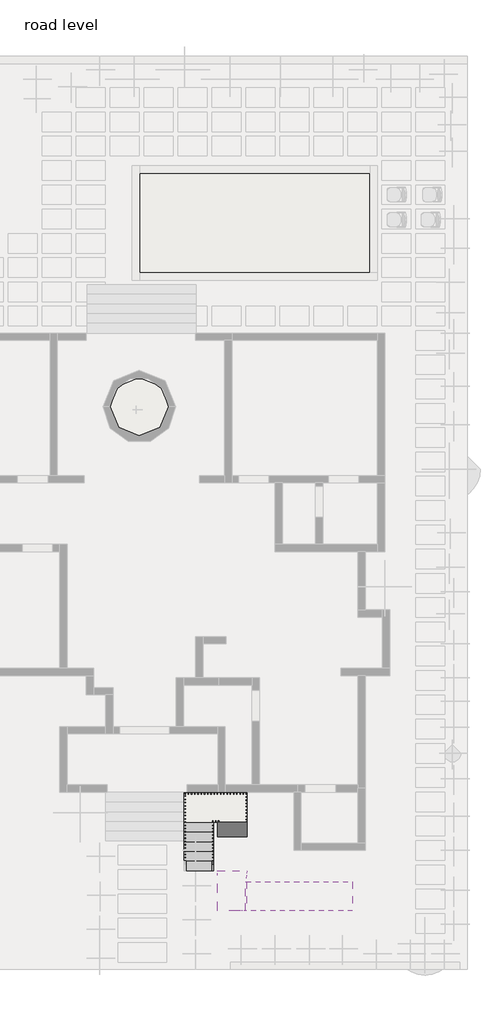
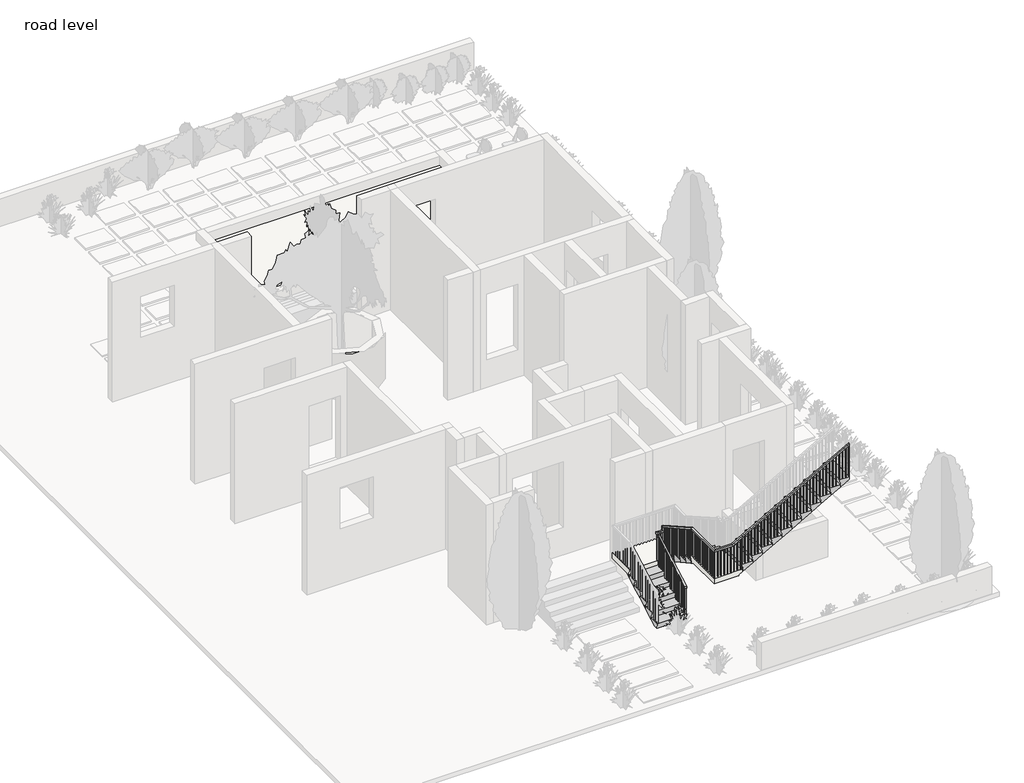
# One storey, part 3 of 5: 7 slabs, 3 stair flights, 1 railing.
"""IFC4 building model written with IfcOpenShell, lengths in millimetres."""

from ifc_helpers import new_model, si_unit, point, frame, frame_2d, origin, origin_with_axes, place, context, project, spatial, polyline, circle_curve, trimmed, segment, composite_curve, outline, extrude, faceted_brep, element, save

model = new_model("IFC4")

# Units and contexts
model_context = context("Model", 3, world=origin())
ifc_project = project(units=[si_unit("LENGTHUNIT", "METRE", prefix="MILLI")], contexts=[model_context])

# Site, building, storey
site = spatial("IfcSite", under=ifc_project)
building = spatial("IfcBuilding", under=site)
storey = spatial("IfcBuildingStorey", under=building, Name="road level", Elevation=0.0)

# Railing
placement = place(None, origin())
element("IfcRailing", 1, ObjectType="Handrail - Rectangular", at=placement, inside=storey, context=model_context, shape_type="SolidModel", body=[
    faceted_brep([(7041.6083823, -2332.334977, 1085.85), (7041.6083823, -2332.334977, 1027.5647478), (7092.4083823, -2332.334977, 1027.5647478), (7092.4083823, -2332.334977, 1085.85), (7041.6083823, -884.534977, 1900.2375), (7041.6083823, -833.734977, 1870.5272478), (7092.4083823, -833.734977, 1870.5272478), (7092.4083823, -884.534977, 1900.2375), (7041.6083823, -884.534977, 1943.1), (7041.6083823, -833.734977, 1892.3), (7092.4083823, -833.734977, 1892.3), (7092.4083823, -884.534977, 1943.1), (7041.6083823, -757.534977, 1943.1), (7041.6083823, -757.534977, 1892.3), (7092.4083823, -808.334977, 1892.3), (7092.4083823, -808.334977, 1943.1), (7168.6083823, -757.534977, 1943.1), (7168.6083823, -757.534977, 1892.3), (7168.6083823, -808.334977, 1892.3), (7168.6083823, -808.334977, 1943.1), (7228.7297505, -757.534977, 1943.1), (7228.7297505, -808.334977, 1943.1), (7279.5297505, -808.334977, 1892.3), (7279.5297505, -757.534977, 1892.3)], [[[0, 1, 2, 3]], [[1, 0, 4, 5]], [[2, 1, 5, 6]], [[3, 2, 6, 7]], [[0, 3, 7, 4]], [[5, 4, 8, 9]], [[6, 5, 9, 10]], [[7, 6, 10, 11]], [[4, 7, 11, 8]], [[9, 8, 12, 13]], [[10, 9, 13, 14]], [[11, 10, 14, 15]], [[8, 11, 15, 12]], [[13, 12, 16, 17]], [[14, 13, 17, 18]], [[15, 14, 18, 19]], [[12, 15, 19, 16]], [[20, 21, 22, 23]], [[17, 16, 20, 23]], [[18, 17, 23, 22]], [[19, 18, 22, 21]], [[16, 19, 21, 20]]]),
    faceted_brep([(7228.7297505, -757.534977, 1943.1), (7279.5297505, -757.534977, 1892.3), (7279.5297505, -808.334977, 1892.3), (7228.7297505, -808.334977, 1943.1), (7228.7297505, -757.534977, 2085.975), (7228.7297505, -808.334977, 2056.2647478), (7279.5297505, -808.334977, 2056.2647478), (7279.5297505, -757.534977, 2085.975)], [[[0, 1, 2, 3]], [[4, 5, 6, 7]], [[1, 0, 4, 7]], [[2, 1, 7, 6]], [[3, 2, 6, 5]], [[0, 3, 5, 4]]]),
    faceted_brep([(7279.5297505, -757.534977, 2085.975), (7279.5297505, -808.334977, 2056.2647478), (7228.7297505, -808.334977, 2056.2647478), (7228.7297505, -757.534977, 2085.975), (7279.5297505, -2332.334977, 2971.8), (7279.5297505, -2345.642092, 2921.0), (7228.7297505, -2345.642092, 2921.0), (7228.7297505, -2332.334977, 2971.8), (7279.5297505, -3537.8093114, 2971.8), (7279.5297505, -3537.8093114, 2921.0), (7228.7297505, -3588.6093114, 2921.0), (7228.7297505, -3588.6093114, 2971.8), (7800.2297505, -3537.8093114, 2971.8), (7813.5368656, -3537.8093114, 2921.0), (7813.5368656, -3588.6093114, 2921.0), (7800.2297505, -3588.6093114, 2971.8), (8105.0297505, -3537.8093114, 3143.25), (8129.9350215, -3537.8093114, 3098.9739627), (8129.9350215, -3588.6093114, 3098.9739627), (8105.0297505, -3588.6093114, 3143.25), (11457.8297505, -3537.8093114, 5029.2), (11457.8297505, -3588.6093114, 5029.2), (11457.8297505, -3588.6093114, 4970.9147478), (11457.8297505, -3537.8093114, 4970.9147478)], [[[0, 1, 2, 3]], [[1, 0, 4, 5]], [[2, 1, 5, 6]], [[3, 2, 6, 7]], [[0, 3, 7, 4]], [[5, 4, 8, 9]], [[6, 5, 9, 10]], [[7, 6, 10, 11]], [[4, 7, 11, 8]], [[9, 8, 12, 13]], [[10, 9, 13, 14]], [[11, 10, 14, 15]], [[8, 11, 15, 12]], [[13, 12, 16, 17]], [[14, 13, 17, 18]], [[15, 14, 18, 19]], [[12, 15, 19, 16]], [[20, 21, 22, 23]], [[17, 16, 20, 23]], [[18, 17, 23, 22]], [[19, 18, 22, 21]], [[16, 19, 21, 20]]]),
    extrude(outline(polyline([(4919.1225603, 11365.7547505), (4908.4069353, 11346.7047505), (3943.35, 11346.7047505), (3943.35, 11365.7547505), (4919.1225603, 11365.7547505)])), frame((0.0, -3572.7343114, 0.0), z_axis=(0.0, 1.0, 0.0), x_axis=(0.0, 0.0, 1.0)), (0.0, 0.0, 1.0), 19.05),
    extrude(outline(polyline([(4861.9725603, 11264.1547505), (4851.2569353, 11245.1047505), (3943.35, 11245.1047505), (3943.35, 11264.1547505), (4861.9725603, 11264.1547505)])), frame((0.0, -3572.7343114, 0.0), z_axis=(0.0, 1.0, 0.0), x_axis=(0.0, 0.0, 1.0)), (0.0, 0.0, 1.0), 19.05),
    extrude(outline(polyline([(4804.8225603, 11162.5547505), (4794.1069353, 11143.5047505), (3943.35, 11143.5047505), (3943.35, 11162.5547505), (4804.8225603, 11162.5547505)])), frame((0.0, -3572.7343114, 0.0), z_axis=(0.0, 1.0, 0.0), x_axis=(0.0, 0.0, 1.0)), (0.0, 0.0, 1.0), 19.05),
    extrude(outline(polyline([(4747.6725603, 11060.9547505), (4736.9569353, 11041.9047505), (3771.9, 11041.9047505), (3771.9, 11060.9547505), (4747.6725603, 11060.9547505)])), frame((0.0, -3572.7343114, 0.0), z_axis=(0.0, 1.0, 0.0), x_axis=(0.0, 0.0, 1.0)), (0.0, 0.0, 1.0), 19.05),
    extrude(outline(polyline([(4690.5225603, 10959.3547505), (4679.8069353, 10940.3047505), (3771.9, 10940.3047505), (3771.9, 10959.3547505), (4690.5225603, 10959.3547505)])), frame((0.0, -3572.7343114, 0.0), z_axis=(0.0, 1.0, 0.0), x_axis=(0.0, 0.0, 1.0)), (0.0, 0.0, 1.0), 19.05),
    extrude(outline(polyline([(4633.3725603, 10857.7547505), (4622.6569353, 10838.7047505), (3771.9, 10838.7047505), (3771.9, 10857.7547505), (4633.3725603, 10857.7547505)])), frame((0.0, -3572.7343114, 0.0), z_axis=(0.0, 1.0, 0.0), x_axis=(0.0, 0.0, 1.0)), (0.0, 0.0, 1.0), 19.05),
    extrude(outline(polyline([(4576.2225603, 10756.1547505), (4565.5069353, 10737.1047505), (3600.45, 10737.1047505), (3600.45, 10756.1547505), (4576.2225603, 10756.1547505)])), frame((0.0, -3572.7343114, 0.0), z_axis=(0.0, 1.0, 0.0), x_axis=(0.0, 0.0, 1.0)), (0.0, 0.0, 1.0), 19.05),
    extrude(outline(polyline([(4519.0725603, 10654.5547505), (4508.3569353, 10635.5047505), (3600.45, 10635.5047505), (3600.45, 10654.5547505), (4519.0725603, 10654.5547505)])), frame((0.0, -3572.7343114, 0.0), z_axis=(0.0, 1.0, 0.0), x_axis=(0.0, 0.0, 1.0)), (0.0, 0.0, 1.0), 19.05),
    extrude(outline(polyline([(4461.9225603, 10552.9547505), (4451.2069353, 10533.9047505), (3600.45, 10533.9047505), (3600.45, 10552.9547505), (4461.9225603, 10552.9547505)])), frame((0.0, -3572.7343114, 0.0), z_axis=(0.0, 1.0, 0.0), x_axis=(0.0, 0.0, 1.0)), (0.0, 0.0, 1.0), 19.05),
    extrude(outline(polyline([(4404.7725603, 10451.3547505), (4394.0569353, 10432.3047505), (3429.0, 10432.3047505), (3429.0, 10451.3547505), (4404.7725603, 10451.3547505)])), frame((0.0, -3572.7343114, 0.0), z_axis=(0.0, 1.0, 0.0), x_axis=(0.0, 0.0, 1.0)), (0.0, 0.0, 1.0), 19.05),
    extrude(outline(polyline([(4347.6225603, 10349.7547505), (4336.9069353, 10330.7047505), (3429.0, 10330.7047505), (3429.0, 10349.7547505), (4347.6225603, 10349.7547505)])), frame((0.0, -3572.7343114, 0.0), z_axis=(0.0, 1.0, 0.0), x_axis=(0.0, 0.0, 1.0)), (0.0, 0.0, 1.0), 19.05),
    extrude(outline(polyline([(4290.4725603, 10248.1547505), (4279.7569353, 10229.1047505), (3429.0, 10229.1047505), (3429.0, 10248.1547505), (4290.4725603, 10248.1547505)])), frame((0.0, -3572.7343114, 0.0), z_axis=(0.0, 1.0, 0.0), x_axis=(0.0, 0.0, 1.0)), (0.0, 0.0, 1.0), 19.05),
    extrude(outline(polyline([(4233.3225603, 10146.5547505), (4222.6069353, 10127.5047505), (3257.55, 10127.5047505), (3257.55, 10146.5547505), (4233.3225603, 10146.5547505)])), frame((0.0, -3572.7343114, 0.0), z_axis=(0.0, 1.0, 0.0), x_axis=(0.0, 0.0, 1.0)), (0.0, 0.0, 1.0), 19.05),
    extrude(outline(polyline([(4176.1725603, 10044.9547505), (4165.4569353, 10025.9047505), (3257.55, 10025.9047505), (3257.55, 10044.9547505), (4176.1725603, 10044.9547505)])), frame((0.0, -3572.7343114, 0.0), z_axis=(0.0, 1.0, 0.0), x_axis=(0.0, 0.0, 1.0)), (0.0, 0.0, 1.0), 19.05),
    extrude(outline(polyline([(4119.0225603, 9943.3547505), (4108.3069353, 9924.3047505), (3257.55, 9924.3047505), (3257.55, 9943.3547505), (4119.0225603, 9943.3547505)])), frame((0.0, -3572.7343114, 0.0), z_axis=(0.0, 1.0, 0.0), x_axis=(0.0, 0.0, 1.0)), (0.0, 0.0, 1.0), 19.05),
    extrude(outline(polyline([(4061.8725603, 9841.7547505), (4051.1569353, 9822.7047505), (3086.1, 9822.7047505), (3086.1, 9841.7547505), (4061.8725603, 9841.7547505)])), frame((0.0, -3572.7343114, 0.0), z_axis=(0.0, 1.0, 0.0), x_axis=(0.0, 0.0, 1.0)), (0.0, 0.0, 1.0), 19.05),
    extrude(outline(polyline([(4004.7225603, 9740.1547505), (3994.0069353, 9721.1047505), (3086.1, 9721.1047505), (3086.1, 9740.1547505), (4004.7225603, 9740.1547505)])), frame((0.0, -3572.7343114, 0.0), z_axis=(0.0, 1.0, 0.0), x_axis=(0.0, 0.0, 1.0)), (0.0, 0.0, 1.0), 19.05),
    extrude(outline(polyline([(3947.5725603, 9638.5547505), (3936.8569353, 9619.5047505), (3086.1, 9619.5047505), (3086.1, 9638.5547505), (3947.5725603, 9638.5547505)])), frame((0.0, -3572.7343114, 0.0), z_axis=(0.0, 1.0, 0.0), x_axis=(0.0, 0.0, 1.0)), (0.0, 0.0, 1.0), 19.05),
    extrude(outline(polyline([(3890.4225603, 9536.9547505), (3879.7069353, 9517.9047505), (2914.65, 9517.9047505), (2914.65, 9536.9547505), (3890.4225603, 9536.9547505)])), frame((0.0, -3572.7343114, 0.0), z_axis=(0.0, 1.0, 0.0), x_axis=(0.0, 0.0, 1.0)), (0.0, 0.0, 1.0), 19.05),
    extrude(outline(polyline([(3833.2725603, 9435.3547505), (3822.5569353, 9416.3047505), (2914.65, 9416.3047505), (2914.65, 9435.3547505), (3833.2725603, 9435.3547505)])), frame((0.0, -3572.7343114, 0.0), z_axis=(0.0, 1.0, 0.0), x_axis=(0.0, 0.0, 1.0)), (0.0, 0.0, 1.0), 19.05),
    extrude(outline(polyline([(3776.1225603, 9333.7547505), (3765.4069353, 9314.7047505), (2914.65, 9314.7047505), (2914.65, 9333.7547505), (3776.1225603, 9333.7547505)])), frame((0.0, -3572.7343114, 0.0), z_axis=(0.0, 1.0, 0.0), x_axis=(0.0, 0.0, 1.0)), (0.0, 0.0, 1.0), 19.05),
    extrude(outline(polyline([(3718.9725603, 9232.1547505), (3708.2569353, 9213.1047505), (2743.2, 9213.1047505), (2743.2, 9232.1547505), (3718.9725603, 9232.1547505)])), frame((0.0, -3572.7343114, 0.0), z_axis=(0.0, 1.0, 0.0), x_axis=(0.0, 0.0, 1.0)), (0.0, 0.0, 1.0), 19.05),
    extrude(outline(polyline([(3661.8225603, 9130.5547505), (3651.1069353, 9111.5047505), (2743.2, 9111.5047505), (2743.2, 9130.5547505), (3661.8225603, 9130.5547505)])), frame((0.0, -3572.7343114, 0.0), z_axis=(0.0, 1.0, 0.0), x_axis=(0.0, 0.0, 1.0)), (0.0, 0.0, 1.0), 19.05),
    extrude(outline(polyline([(3604.6725603, 9028.9547505), (3593.9569353, 9009.9047505), (2743.2, 9009.9047505), (2743.2, 9028.9547505), (3604.6725603, 9028.9547505)])), frame((0.0, -3572.7343114, 0.0), z_axis=(0.0, 1.0, 0.0), x_axis=(0.0, 0.0, 1.0)), (0.0, 0.0, 1.0), 19.05),
    extrude(outline(polyline([(3547.5225603, 8927.3547505), (3536.8069353, 8908.3047505), (2571.75, 8908.3047505), (2571.75, 8927.3547505), (3547.5225603, 8927.3547505)])), frame((0.0, -3572.7343114, 0.0), z_axis=(0.0, 1.0, 0.0), x_axis=(0.0, 0.0, 1.0)), (0.0, 0.0, 1.0), 19.05),
    extrude(outline(polyline([(3490.3725603, 8825.7547505), (3479.6569353, 8806.7047505), (2571.75, 8806.7047505), (2571.75, 8825.7547505), (3490.3725603, 8825.7547505)])), frame((0.0, -3572.7343114, 0.0), z_axis=(0.0, 1.0, 0.0), x_axis=(0.0, 0.0, 1.0)), (0.0, 0.0, 1.0), 19.05),
    extrude(outline(polyline([(3433.2225603, 8724.1547505), (3422.5069353, 8705.1047505), (2571.75, 8705.1047505), (2571.75, 8724.1547505), (3433.2225603, 8724.1547505)])), frame((0.0, -3572.7343114, 0.0), z_axis=(0.0, 1.0, 0.0), x_axis=(0.0, 0.0, 1.0)), (0.0, 0.0, 1.0), 19.05),
    extrude(outline(polyline([(3376.0725603, 8622.5547505), (3365.3569353, 8603.5047505), (2400.3, 8603.5047505), (2400.3, 8622.5547505), (3376.0725603, 8622.5547505)])), frame((0.0, -3572.7343114, 0.0), z_axis=(0.0, 1.0, 0.0), x_axis=(0.0, 0.0, 1.0)), (0.0, 0.0, 1.0), 19.05),
    extrude(outline(polyline([(3318.9225603, 8520.9547505), (3308.2069353, 8501.9047505), (2400.3, 8501.9047505), (2400.3, 8520.9547505), (3318.9225603, 8520.9547505)])), frame((0.0, -3572.7343114, 0.0), z_axis=(0.0, 1.0, 0.0), x_axis=(0.0, 0.0, 1.0)), (0.0, 0.0, 1.0), 19.05),
    extrude(outline(polyline([(3261.7725603, 8419.3547505), (3251.0569353, 8400.3047505), (2400.3, 8400.3047505), (2400.3, 8419.3547505), (3261.7725603, 8419.3547505)])), frame((0.0, -3572.7343114, 0.0), z_axis=(0.0, 1.0, 0.0), x_axis=(0.0, 0.0, 1.0)), (0.0, 0.0, 1.0), 19.05),
    extrude(outline(polyline([(3204.6225603, 8317.7547505), (3193.9069353, 8298.7047505), (2228.85, 8298.7047505), (2228.85, 8317.7547505), (3204.6225603, 8317.7547505)])), frame((0.0, -3572.7343114, 0.0), z_axis=(0.0, 1.0, 0.0), x_axis=(0.0, 0.0, 1.0)), (0.0, 0.0, 1.0), 19.05),
    extrude(outline(polyline([(3147.4725603, 8216.1547505), (3136.7569353, 8197.1047505), (2228.85, 8197.1047505), (2228.85, 8216.1547505), (3147.4725603, 8216.1547505)])), frame((0.0, -3572.7343114, 0.0), z_axis=(0.0, 1.0, 0.0), x_axis=(0.0, 0.0, 1.0)), (0.0, 0.0, 1.0), 19.05),
    extrude(outline(polyline([(3068.8913103, 8076.4547505), (3058.1756853, 8057.4047505), (2057.4, 8057.4047505), (2057.4, 8076.4547505), (3068.8913103, 8076.4547505)])), frame((0.0, -3572.7343114, 0.0), z_axis=(0.0, 1.0, 0.0), x_axis=(0.0, 0.0, 1.0)), (0.0, 0.0, 1.0), 19.05),
    extrude(outline(polyline([(3011.7413103, 7974.8547505), (3001.0256853, 7955.8047505), (2057.4, 7955.8047505), (2057.4, 7974.8547505), (3011.7413103, 7974.8547505)])), frame((0.0, -3572.7343114, 0.0), z_axis=(0.0, 1.0, 0.0), x_axis=(0.0, 0.0, 1.0)), (0.0, 0.0, 1.0), 19.05),
    extrude(outline(polyline([(2954.5913103, 7873.2547505), (2943.8756853, 7854.2047505), (2057.4, 7854.2047505), (2057.4, 7873.2547505), (2954.5913103, 7873.2547505)])), frame((0.0, -3572.7343114, 0.0), z_axis=(0.0, 1.0, 0.0), x_axis=(0.0, 0.0, 1.0)), (0.0, 0.0, 1.0), 19.05),
    extrude(outline(polyline([(7752.6047505, -3572.7343114), (7752.6047505, -3553.6843114), (7771.6547505, -3553.6843114), (7771.6547505, -3572.7343114), (7752.6047505, -3572.7343114)])), frame((0.0, 0.0, 2057.4), z_axis=(0.0, 0.0, 1.0), x_axis=(1.0, 0.0, 0.0)), (0.0, 0.0, 1.0), 863.6),
    extrude(outline(polyline([(7651.0047505, -3572.7343114), (7651.0047505, -3553.6843114), (7670.0547505, -3553.6843114), (7670.0547505, -3572.7343114), (7651.0047505, -3572.7343114)])), frame((0.0, 0.0, 2057.4), z_axis=(0.0, 0.0, 1.0), x_axis=(1.0, 0.0, 0.0)), (0.0, 0.0, 1.0), 863.6),
    extrude(outline(polyline([(7549.4047505, -3572.7343114), (7549.4047505, -3553.6843114), (7568.4547505, -3553.6843114), (7568.4547505, -3572.7343114), (7549.4047505, -3572.7343114)])), frame((0.0, 0.0, 2057.4), z_axis=(0.0, 0.0, 1.0), x_axis=(1.0, 0.0, 0.0)), (0.0, 0.0, 1.0), 863.6),
    extrude(outline(polyline([(7447.8047505, -3572.7343114), (7447.8047505, -3553.6843114), (7466.8547505, -3553.6843114), (7466.8547505, -3572.7343114), (7447.8047505, -3572.7343114)])), frame((0.0, 0.0, 2057.4), z_axis=(0.0, 0.0, 1.0), x_axis=(1.0, 0.0, 0.0)), (0.0, 0.0, 1.0), 863.6),
    extrude(outline(polyline([(7346.2047505, -3572.7343114), (7346.2047505, -3553.6843114), (7365.2547505, -3553.6843114), (7365.2547505, -3572.7343114), (7346.2047505, -3572.7343114)])), frame((0.0, 0.0, 2057.4), z_axis=(0.0, 0.0, 1.0), x_axis=(1.0, 0.0, 0.0)), (0.0, 0.0, 1.0), 863.6),
    extrude(outline(polyline([(7244.6047505, -3542.009977), (7263.6547505, -3542.009977), (7263.6547505, -3561.059977), (7244.6047505, -3561.059977), (7244.6047505, -3542.009977)])), frame((0.0, 0.0, 2057.4), z_axis=(0.0, 0.0, 1.0), x_axis=(1.0, 0.0, 0.0)), (0.0, 0.0, 1.0), 863.6),
    extrude(outline(polyline([(7244.6047505, -3440.409977), (7263.6547505, -3440.409977), (7263.6547505, -3459.459977), (7244.6047505, -3459.459977), (7244.6047505, -3440.409977)])), frame((0.0, 0.0, 2057.4), z_axis=(0.0, 0.0, 1.0), x_axis=(1.0, 0.0, 0.0)), (0.0, 0.0, 1.0), 863.6),
    extrude(outline(polyline([(7244.6047505, -3338.809977), (7263.6547505, -3338.809977), (7263.6547505, -3357.859977), (7244.6047505, -3357.859977), (7244.6047505, -3338.809977)])), frame((0.0, 0.0, 2057.4), z_axis=(0.0, 0.0, 1.0), x_axis=(1.0, 0.0, 0.0)), (0.0, 0.0, 1.0), 863.6),
    extrude(outline(polyline([(7244.6047505, -3237.209977), (7263.6547505, -3237.209977), (7263.6547505, -3256.259977), (7244.6047505, -3256.259977), (7244.6047505, -3237.209977)])), frame((0.0, 0.0, 2057.4), z_axis=(0.0, 0.0, 1.0), x_axis=(1.0, 0.0, 0.0)), (0.0, 0.0, 1.0), 863.6),
    extrude(outline(polyline([(7244.6047505, -3135.609977), (7263.6547505, -3135.609977), (7263.6547505, -3154.659977), (7244.6047505, -3154.659977), (7244.6047505, -3135.609977)])), frame((0.0, 0.0, 2057.4), z_axis=(0.0, 0.0, 1.0), x_axis=(1.0, 0.0, 0.0)), (0.0, 0.0, 1.0), 863.6),
    extrude(outline(polyline([(7244.6047505, -3034.009977), (7263.6547505, -3034.009977), (7263.6547505, -3053.059977), (7244.6047505, -3053.059977), (7244.6047505, -3034.009977)])), frame((0.0, 0.0, 2057.4), z_axis=(0.0, 0.0, 1.0), x_axis=(1.0, 0.0, 0.0)), (0.0, 0.0, 1.0), 863.6),
    extrude(outline(polyline([(7244.6047505, -2932.409977), (7263.6547505, -2932.409977), (7263.6547505, -2951.459977), (7244.6047505, -2951.459977), (7244.6047505, -2932.409977)])), frame((0.0, 0.0, 2057.4), z_axis=(0.0, 0.0, 1.0), x_axis=(1.0, 0.0, 0.0)), (0.0, 0.0, 1.0), 863.6),
    extrude(outline(polyline([(7244.6047505, -2830.809977), (7263.6547505, -2830.809977), (7263.6547505, -2849.859977), (7244.6047505, -2849.859977), (7244.6047505, -2830.809977)])), frame((0.0, 0.0, 2057.4), z_axis=(0.0, 0.0, 1.0), x_axis=(1.0, 0.0, 0.0)), (0.0, 0.0, 1.0), 863.6),
    extrude(outline(polyline([(7244.6047505, -2729.209977), (7263.6547505, -2729.209977), (7263.6547505, -2748.259977), (7244.6047505, -2748.259977), (7244.6047505, -2729.209977)])), frame((0.0, 0.0, 2057.4), z_axis=(0.0, 0.0, 1.0), x_axis=(1.0, 0.0, 0.0)), (0.0, 0.0, 1.0), 863.6),
    extrude(outline(polyline([(7244.6047505, -2627.609977), (7263.6547505, -2627.609977), (7263.6547505, -2646.659977), (7244.6047505, -2646.659977), (7244.6047505, -2627.609977)])), frame((0.0, 0.0, 2057.4), z_axis=(0.0, 0.0, 1.0), x_axis=(1.0, 0.0, 0.0)), (0.0, 0.0, 1.0), 863.6),
    extrude(outline(polyline([(7244.6047505, -2526.009977), (7263.6547505, -2526.009977), (7263.6547505, -2545.059977), (7244.6047505, -2545.059977), (7244.6047505, -2526.009977)])), frame((0.0, 0.0, 2057.4), z_axis=(0.0, 0.0, 1.0), x_axis=(1.0, 0.0, 0.0)), (0.0, 0.0, 1.0), 863.6),
    extrude(outline(polyline([(7244.6047505, -2424.409977), (7263.6547505, -2424.409977), (7263.6547505, -2443.459977), (7244.6047505, -2443.459977), (7244.6047505, -2424.409977)])), frame((0.0, 0.0, 2057.4), z_axis=(0.0, 0.0, 1.0), x_axis=(1.0, 0.0, 0.0)), (0.0, 0.0, 1.0), 863.6),
    extrude(outline(polyline([(-2316.459977, 2904.5850603), (-2297.409977, 2893.8694353), (-2297.409977, 1885.95), (-2316.459977, 1885.95), (-2316.459977, 2904.5850603)])), frame((7244.6047505, 0.0, 0.0), z_axis=(1.0, 0.0, 0.0), x_axis=(0.0, 1.0, 0.0)), (0.0, 0.0, 1.0), 19.05),
    extrude(outline(polyline([(-2214.859977, 2847.4350603), (-2195.809977, 2836.7194353), (-2195.809977, 1885.95), (-2214.859977, 1885.95), (-2214.859977, 2847.4350603)])), frame((7244.6047505, 0.0, 0.0), z_axis=(1.0, 0.0, 0.0), x_axis=(0.0, 1.0, 0.0)), (0.0, 0.0, 1.0), 19.05),
    extrude(outline(polyline([(-2113.259977, 2790.2850603), (-2094.209977, 2779.5694353), (-2094.209977, 1885.95), (-2113.259977, 1885.95), (-2113.259977, 2790.2850603)])), frame((7244.6047505, 0.0, 0.0), z_axis=(1.0, 0.0, 0.0), x_axis=(0.0, 1.0, 0.0)), (0.0, 0.0, 1.0), 19.05),
    extrude(outline(polyline([(-2011.659977, 2733.1350603), (-1992.609977, 2722.4194353), (-1992.609977, 1714.5), (-2011.659977, 1714.5), (-2011.659977, 2733.1350603)])), frame((7244.6047505, 0.0, 0.0), z_axis=(1.0, 0.0, 0.0), x_axis=(0.0, 1.0, 0.0)), (0.0, 0.0, 1.0), 19.05),
    extrude(outline(polyline([(-1910.059977, 2675.9850603), (-1891.009977, 2665.2694353), (-1891.009977, 1714.5), (-1910.059977, 1714.5), (-1910.059977, 2675.9850603)])), frame((7244.6047505, 0.0, 0.0), z_axis=(1.0, 0.0, 0.0), x_axis=(0.0, 1.0, 0.0)), (0.0, 0.0, 1.0), 19.05),
    extrude(outline(polyline([(-1808.459977, 2618.8350603), (-1789.409977, 2608.1194353), (-1789.409977, 1714.5), (-1808.459977, 1714.5), (-1808.459977, 2618.8350603)])), frame((7244.6047505, 0.0, 0.0), z_axis=(1.0, 0.0, 0.0), x_axis=(0.0, 1.0, 0.0)), (0.0, 0.0, 1.0), 19.05),
    extrude(outline(polyline([(-1706.859977, 2561.6850603), (-1687.809977, 2550.9694353), (-1687.809977, 1543.05), (-1706.859977, 1543.05), (-1706.859977, 2561.6850603)])), frame((7244.6047505, 0.0, 0.0), z_axis=(1.0, 0.0, 0.0), x_axis=(0.0, 1.0, 0.0)), (0.0, 0.0, 1.0), 19.05),
    extrude(outline(polyline([(-1605.259977, 2504.5350603), (-1586.209977, 2493.8194353), (-1586.209977, 1543.05), (-1605.259977, 1543.05), (-1605.259977, 2504.5350603)])), frame((7244.6047505, 0.0, 0.0), z_axis=(1.0, 0.0, 0.0), x_axis=(0.0, 1.0, 0.0)), (0.0, 0.0, 1.0), 19.05),
    extrude(outline(polyline([(-1503.659977, 2447.3850603), (-1484.609977, 2436.6694353), (-1484.609977, 1543.05), (-1503.659977, 1543.05), (-1503.659977, 2447.3850603)])), frame((7244.6047505, 0.0, 0.0), z_axis=(1.0, 0.0, 0.0), x_axis=(0.0, 1.0, 0.0)), (0.0, 0.0, 1.0), 19.05),
    extrude(outline(polyline([(-1402.059977, 2390.2350603), (-1383.009977, 2379.5194353), (-1383.009977, 1371.6), (-1402.059977, 1371.6), (-1402.059977, 2390.2350603)])), frame((7244.6047505, 0.0, 0.0), z_axis=(1.0, 0.0, 0.0), x_axis=(0.0, 1.0, 0.0)), (0.0, 0.0, 1.0), 19.05),
    extrude(outline(polyline([(-1300.459977, 2333.0850603), (-1281.409977, 2322.3694353), (-1281.409977, 1371.6), (-1300.459977, 1371.6), (-1300.459977, 2333.0850603)])), frame((7244.6047505, 0.0, 0.0), z_axis=(1.0, 0.0, 0.0), x_axis=(0.0, 1.0, 0.0)), (0.0, 0.0, 1.0), 19.05),
    extrude(outline(polyline([(-1198.859977, 2275.9350603), (-1179.809977, 2265.2194353), (-1179.809977, 1371.6), (-1198.859977, 1371.6), (-1198.859977, 2275.9350603)])), frame((7244.6047505, 0.0, 0.0), z_axis=(1.0, 0.0, 0.0), x_axis=(0.0, 1.0, 0.0)), (0.0, 0.0, 1.0), 19.05),
    extrude(outline(polyline([(-1097.259977, 2218.7850603), (-1078.209977, 2208.0694353), (-1078.209977, 1200.15), (-1097.259977, 1200.15), (-1097.259977, 2218.7850603)])), frame((7244.6047505, 0.0, 0.0), z_axis=(1.0, 0.0, 0.0), x_axis=(0.0, 1.0, 0.0)), (0.0, 0.0, 1.0), 19.05),
    extrude(outline(polyline([(-995.659977, 2161.6350603), (-976.609977, 2150.9194353), (-976.609977, 1200.15), (-995.659977, 1200.15), (-995.659977, 2161.6350603)])), frame((7244.6047505, 0.0, 0.0), z_axis=(1.0, 0.0, 0.0), x_axis=(0.0, 1.0, 0.0)), (0.0, 0.0, 1.0), 19.05),
    extrude(outline(polyline([(-894.059977, 2104.4850603), (-875.009977, 2093.7694353), (-875.009977, 1200.15), (-894.059977, 1200.15), (-894.059977, 2104.4850603)])), frame((7244.6047505, 0.0, 0.0), z_axis=(1.0, 0.0, 0.0), x_axis=(0.0, 1.0, 0.0)), (0.0, 0.0, 1.0), 19.05),
    extrude(outline(polyline([(7159.0833823, -792.459977), (7159.0833823, -773.409977), (7178.1333823, -773.409977), (7178.1333823, -792.459977), (7159.0833823, -792.459977)])), frame((0.0, 0.0, 1028.7), z_axis=(0.0, 0.0, 1.0), x_axis=(1.0, 0.0, 0.0)), (0.0, 0.0, 1.0), 863.6),
    extrude(outline(polyline([(7076.5333823, -817.859977), (7057.4833823, -817.859977), (7057.4833823, -798.809977), (7076.5333823, -798.809977), (7076.5333823, -817.859977)])), frame((0.0, 0.0, 1028.7), z_axis=(0.0, 0.0, 1.0), x_axis=(1.0, 0.0, 0.0)), (0.0, 0.0, 1.0), 863.6),
    extrude(outline(polyline([(-919.459977, 1822.3069353), (-900.409977, 1833.0225603), (-900.409977, 857.25), (-919.459977, 857.25), (-919.459977, 1822.3069353)])), frame((7057.4833823, 0.0, 0.0), z_axis=(1.0, 0.0, 0.0), x_axis=(0.0, 1.0, 0.0)), (0.0, 0.0, 1.0), 19.05),
    extrude(outline(polyline([(-1021.059977, 1765.1569353), (-1002.009977, 1775.8725603), (-1002.009977, 857.25), (-1021.059977, 857.25), (-1021.059977, 1765.1569353)])), frame((7057.4833823, 0.0, 0.0), z_axis=(1.0, 0.0, 0.0), x_axis=(0.0, 1.0, 0.0)), (0.0, 0.0, 1.0), 19.05),
    extrude(outline(polyline([(-1122.659977, 1708.0069353), (-1103.609977, 1718.7225603), (-1103.609977, 857.25), (-1122.659977, 857.25), (-1122.659977, 1708.0069353)])), frame((7057.4833823, 0.0, 0.0), z_axis=(1.0, 0.0, 0.0), x_axis=(0.0, 1.0, 0.0)), (0.0, 0.0, 1.0), 19.05),
    extrude(outline(polyline([(-1224.259977, 1650.8569353), (-1205.209977, 1661.5725603), (-1205.209977, 685.8), (-1224.259977, 685.8), (-1224.259977, 1650.8569353)])), frame((7057.4833823, 0.0, 0.0), z_axis=(1.0, 0.0, 0.0), x_axis=(0.0, 1.0, 0.0)), (0.0, 0.0, 1.0), 19.05),
    extrude(outline(polyline([(-1325.859977, 1593.7069353), (-1306.809977, 1604.4225603), (-1306.809977, 685.8), (-1325.859977, 685.8), (-1325.859977, 1593.7069353)])), frame((7057.4833823, 0.0, 0.0), z_axis=(1.0, 0.0, 0.0), x_axis=(0.0, 1.0, 0.0)), (0.0, 0.0, 1.0), 19.05),
    extrude(outline(polyline([(-1427.459977, 1536.5569353), (-1408.409977, 1547.2725603), (-1408.409977, 685.8), (-1427.459977, 685.8), (-1427.459977, 1536.5569353)])), frame((7057.4833823, 0.0, 0.0), z_axis=(1.0, 0.0, 0.0), x_axis=(0.0, 1.0, 0.0)), (0.0, 0.0, 1.0), 19.05),
    extrude(outline(polyline([(-1529.059977, 1479.4069353), (-1510.009977, 1490.1225603), (-1510.009977, 514.35), (-1529.059977, 514.35), (-1529.059977, 1479.4069353)])), frame((7057.4833823, 0.0, 0.0), z_axis=(1.0, 0.0, 0.0), x_axis=(0.0, 1.0, 0.0)), (0.0, 0.0, 1.0), 19.05),
    extrude(outline(polyline([(-1630.659977, 1422.2569353), (-1611.609977, 1432.9725603), (-1611.609977, 514.35), (-1630.659977, 514.35), (-1630.659977, 1422.2569353)])), frame((7057.4833823, 0.0, 0.0), z_axis=(1.0, 0.0, 0.0), x_axis=(0.0, 1.0, 0.0)), (0.0, 0.0, 1.0), 19.05),
    extrude(outline(polyline([(-1732.259977, 1365.1069353), (-1713.209977, 1375.8225603), (-1713.209977, 514.35), (-1732.259977, 514.35), (-1732.259977, 1365.1069353)])), frame((7057.4833823, 0.0, 0.0), z_axis=(1.0, 0.0, 0.0), x_axis=(0.0, 1.0, 0.0)), (0.0, 0.0, 1.0), 19.05),
    extrude(outline(polyline([(-1833.859977, 1307.9569353), (-1814.809977, 1318.6725603), (-1814.809977, 342.9), (-1833.859977, 342.9), (-1833.859977, 1307.9569353)])), frame((7057.4833823, 0.0, 0.0), z_axis=(1.0, 0.0, 0.0), x_axis=(0.0, 1.0, 0.0)), (0.0, 0.0, 1.0), 19.05),
    extrude(outline(polyline([(-1935.459977, 1250.8069353), (-1916.409977, 1261.5225603), (-1916.409977, 342.9), (-1935.459977, 342.9), (-1935.459977, 1250.8069353)])), frame((7057.4833823, 0.0, 0.0), z_axis=(1.0, 0.0, 0.0), x_axis=(0.0, 1.0, 0.0)), (0.0, 0.0, 1.0), 19.05),
    extrude(outline(polyline([(-2037.059977, 1193.6569353), (-2018.009977, 1204.3725603), (-2018.009977, 342.9), (-2037.059977, 342.9), (-2037.059977, 1193.6569353)])), frame((7057.4833823, 0.0, 0.0), z_axis=(1.0, 0.0, 0.0), x_axis=(0.0, 1.0, 0.0)), (0.0, 0.0, 1.0), 19.05),
    extrude(outline(polyline([(-2138.659977, 1136.5069353), (-2119.609977, 1147.2225603), (-2119.609977, 171.45), (-2138.659977, 171.45), (-2138.659977, 1136.5069353)])), frame((7057.4833823, 0.0, 0.0), z_axis=(1.0, 0.0, 0.0), x_axis=(0.0, 1.0, 0.0)), (0.0, 0.0, 1.0), 19.05),
    extrude(outline(polyline([(-2240.259977, 1079.3569353), (-2221.209977, 1090.0725603), (-2221.209977, 171.45), (-2240.259977, 171.45), (-2240.259977, 1079.3569353)])), frame((7057.4833823, 0.0, 0.0), z_axis=(1.0, 0.0, 0.0), x_axis=(0.0, 1.0, 0.0)), (0.0, 0.0, 1.0), 19.05),
    extrude(outline(polyline([(3090.3225603, 8114.5547505), (3079.6069353, 8095.5047505), (2057.4, 8095.5047505), (2057.4, 8114.5547505), (3090.3225603, 8114.5547505)])), frame((0.0, -3572.7343114, 0.0), z_axis=(0.0, 1.0, 0.0), x_axis=(0.0, 0.0, 1.0)), (0.0, 0.0, 1.0), 19.05),
    extrude(outline(polyline([(7244.6047505, -3553.6843114), (7263.6547505, -3553.6843114), (7263.6547505, -3572.7343114), (7244.6047505, -3572.7343114), (7244.6047505, -3553.6843114)])), frame((0.0, 0.0, 2057.4), z_axis=(0.0, 0.0, 1.0), x_axis=(1.0, 0.0, 0.0)), (0.0, 0.0, 1.0), 863.6),
    extrude(outline(polyline([(-2341.859977, 2918.8725603), (-2322.809977, 2908.1569353), (-2322.809977, 2057.4), (-2341.859977, 2057.4), (-2341.859977, 2918.8725603)])), frame((7244.6047505, 0.0, 0.0), z_axis=(1.0, 0.0, 0.0), x_axis=(0.0, 1.0, 0.0)), (0.0, 0.0, 1.0), 19.05),
    extrude(outline(polyline([(7244.6047505, -792.459977), (7244.6047505, -773.409977), (7263.6547505, -773.409977), (7263.6547505, -792.459977), (7244.6047505, -792.459977)])), frame((0.0, 0.0, 1028.7), z_axis=(0.0, 0.0, 1.0), x_axis=(1.0, 0.0, 0.0)), (0.0, 0.0, 1.0), 863.6),
    extrude(outline(polyline([(7076.5333823, -792.459977), (7057.4833823, -792.459977), (7057.4833823, -773.409977), (7076.5333823, -773.409977), (7076.5333823, -792.459977)])), frame((0.0, 0.0, 1028.7), z_axis=(0.0, 0.0, 1.0), x_axis=(1.0, 0.0, 0.0)), (0.0, 0.0, 1.0), 863.6),
    extrude(outline(polyline([(4970.9147478, 11457.8297505), (4960.1991228, 11438.7797505), (3943.35, 11438.7797505), (3943.35, 11457.8297505), (4970.9147478, 11457.8297505)])), frame((0.0, -3572.7343114, 0.0), z_axis=(0.0, 1.0, 0.0), x_axis=(0.0, 0.0, 1.0)), (0.0, 0.0, 1.0), 19.05),
    extrude(outline(polyline([(-2332.334977, 1027.5647478), (-2313.284977, 1038.2803728), (-2313.284977, 171.45), (-2332.334977, 171.45), (-2332.334977, 1027.5647478)])), frame((7057.4833823, 0.0, 0.0), z_axis=(1.0, 0.0, 0.0), x_axis=(0.0, 1.0, 0.0)), (0.0, 0.0, 1.0), 19.05),
])

# Slabs
element("IfcSlab", 2, at=placement, inside=storey, context=model_context, shape_type="SweptSolid", body=[
    extrude(outline(polyline([(12246.4512825, 16197.9906886), (4540.3394971, 16197.9906886), (4540.3394971, 19779.3906886), (12246.4512825, 19779.3906886), (12246.4512825, 16197.9906886)])), frame((0.0, 0.0, -1829.9170041), z_axis=(0.0, 0.0, 1.0), x_axis=(1.0, 0.0, 0.0)), (0.0, 0.0, 1.0), 152.4),
])
element("IfcSlab", 3, at=placement, inside=storey, context=model_context, shape_type="SweptSolid", body=[
    extrude(outline(polyline([(12007.9394971, 16426.5906886), (4768.9394971, 16426.5906886), (4768.9394971, 19550.7906886), (12007.9394971, 19550.7906886), (12007.9394971, 16426.5906886)])), frame((0.0, 0.0, -1524.0), z_axis=(0.0, 0.0, 1.0), x_axis=(1.0, 0.0, 0.0)), (0.0, 0.0, 1.0), 1524.0),
])
element("IfcSlab", 4, at=placement, inside=storey, context=model_context, shape_type="SweptSolid", body=[
    extrude(outline(composite_curve([segment(trimmed(circle_curve(frame_2d((4765.7160064, 12224.5614263)), 914.4), [point((3851.3160064, 12224.5614263))], [point((5680.1160064, 12224.5614263))], False, "CARTESIAN"), True, "CONTINUOUS"), segment(trimmed(circle_curve(frame_2d((4765.7160064, 12224.5614263)), 914.4), [point((5680.1160064, 12224.5614263))], [point((3851.3160064, 12224.5614263))], False, "CARTESIAN"), True, "CONTINUOUS")], self_intersect=False)), origin_with_axes(), (0.0, 0.0, 1.0), 152.4),
])
element("IfcSlab", 5, at=placement, inside=storey, context=model_context, shape_type="SweptSolid", body=[
    extrude(outline(composite_curve([segment(trimmed(circle_curve(frame_2d((4765.7160064, 12224.5614263)), 914.4), [point((3851.3160064, 12224.5614263))], [point((5680.1160064, 12224.5614263))], False, "CARTESIAN"), True, "CONTINUOUS"), segment(trimmed(circle_curve(frame_2d((4765.7160064, 12224.5614263)), 914.4), [point((5680.1160064, 12224.5614263))], [point((3851.3160064, 12224.5614263))], False, "CARTESIAN"), True, "CONTINUOUS")], self_intersect=False)), origin_with_axes(), (0.0, 0.0, 1.0), 152.4),
])
element("IfcSlab", 6, at=placement, inside=storey, context=model_context, shape_type="SweptSolid", body=[
    extrude(outline(composite_curve([segment(trimmed(circle_curve(frame_2d((4764.1174977, 12217.8800926)), 914.4), [point((3849.7174977, 12217.8800926))], [point((5678.5174977, 12217.8800926))], False, "CARTESIAN"), True, "CONTINUOUS"), segment(trimmed(circle_curve(frame_2d((4764.1174977, 12217.8800926)), 914.4), [point((5678.5174977, 12217.8800926))], [point((3849.7174977, 12217.8800926))], False, "CARTESIAN"), True, "CONTINUOUS")], self_intersect=False)), frame((0.0, 0.0, 152.4), z_axis=(0.0, 0.0, 1.0), x_axis=(1.0, 0.0, 0.0)), (0.0, 0.0, 1.0), 152.4),
])
element("IfcSlab", 7, ObjectType="7\" Thickness", at=placement, inside=storey, context=model_context, shape_type="Brep", body=[
    faceted_brep([(7092.4083823, -808.334977, 1028.7), (6178.0083823, -808.334977, 1028.7), (6178.0083823, -789.284977, 857.25), (7092.4083823, -789.284977, 857.25), (7228.7297505, -808.334977, 1028.7), (7228.7297505, -827.384977, 1028.7), (8143.1297505, -827.384977, 1028.7), (8143.1297505, -808.334977, 1028.7), (8143.1297505, -640.8188708, 1028.7), (8143.1297505, 106.065023, 1028.7), (6178.0083823, 106.065023, 1028.7), (6178.0083823, -671.0510832, 1028.7), (6178.0083823, -789.284977, 784.3934347), (7092.4083823, -789.284977, 784.3934347), (7092.4083823, -789.284977, 850.9), (7092.4083823, -808.334977, 850.9), (7228.7297505, -808.334977, 850.9), (7228.7297505, -808.334977, 945.1278097), (7228.7297505, -827.384977, 955.8434347), (8143.1297505, -827.384977, 955.8434347), (8143.1297505, -808.334977, 945.1278097), (8143.1297505, -640.8188708, 850.9), (8143.1297505, 106.065023, 850.9), (6178.0083823, 106.065023, 850.9), (6178.0083823, -671.0510832, 850.9), (7228.7297505, -640.8188708, 850.9), (7092.4083823, -671.0510832, 850.9)], [[[0, 1, 2, 3]], [[0, 4, 5, 6, 7, 8, 9, 10, 11, 1]], [[3, 2, 12, 13, 14]], [[0, 3, 14, 15]], [[4, 0, 15, 16, 17]], [[5, 4, 17, 18]], [[6, 5, 18, 19]], [[7, 6, 19, 20]], [[7, 20, 21, 22, 9, 8]], [[10, 9, 22, 23]], [[2, 1, 11, 10, 23, 24, 12]], [[25, 16, 15, 14, 26, 24, 23, 22, 21]], [[16, 25, 17]], [[24, 26, 13, 12]], [[26, 14, 13]], [[25, 21, 20, 19, 18, 17]]]),
])
element("IfcSlab", 8, ObjectType="7\" Thickness", at=placement, inside=storey, context=model_context, shape_type="Brep", body=[
    faceted_brep([(7228.7297505, -2332.334977, 2057.4), (8143.1297505, -2332.334977, 2057.4), (8141.0067336, -2351.384977, 1885.95), (7228.7297505, -2351.384977, 1885.95), (8105.0297505, -3588.6093114, 2057.4), (8124.0797505, -3588.6093114, 2057.4), (8124.0797505, -2674.2093114, 2057.4), (8105.0297505, -2674.2093114, 2057.4), (7228.7297505, -2469.6188708, 2057.4), (7228.7297505, -3588.6093114, 2057.4), (8003.1249379, -3588.6093114, 2057.4), (8141.0067336, -2351.384977, 1813.0934347), (7228.7297505, -2351.384977, 1813.0934347), (7228.7297505, -2469.6188708, 1879.6), (7228.7297505, -3588.6093114, 1879.6), (7937.5136443, -3588.6093114, 1879.6), (8003.1249379, -3588.6093114, 1879.6), (8003.1249379, -3588.6093114, 1916.5063526), (8105.0297505, -3588.6093114, 1973.8278097), (8124.0797505, -3588.6093114, 1984.5434347), (8124.0797505, -2674.2093114, 1984.5434347), (8105.0297505, -2674.2093114, 1973.8278097), (8127.8302214, -2469.6188708, 1879.6)], [[[0, 1, 2, 3]], [[4, 5, 6, 7, 1, 0, 8, 9, 10]], [[3, 2, 11, 12]], [[0, 3, 12, 13, 14, 9, 8]], [[9, 14, 15, 16, 17, 18, 4, 10]], [[5, 4, 18, 19]], [[6, 5, 19, 20]], [[7, 6, 20, 21]], [[2, 1, 7, 21, 17, 16, 22, 11]], [[13, 22, 16, 15, 14]], [[22, 13, 12, 11]], [[17, 21, 20, 19, 18]]]),
])

# Stair flights
element("IfcStairFlight", 9, ObjectType="3/4\" Nosing", at=placement, inside=storey, context=model_context, shape_type="Brep", body=[
    faceted_brep([(7092.4083823, -2332.334977, 171.45), (6178.0083823, -2332.334977, 171.45), (6178.0083823, -2313.284977, 0.0), (7092.4083823, -2313.284977, 0.0), (7092.4083823, -2008.484977, 171.45), (6178.0083823, -2008.484977, 171.45), (6178.0083823, -2008.484977, 98.5934347), (6178.0083823, -2183.7621943, 0.0), (7092.4083823, -2183.7621943, 0.0), (7092.4083823, -2008.484977, 98.5934347), (6178.0083823, -2027.534977, 342.9), (7092.4083823, -2027.534977, 342.9), (7092.4083823, -1703.684977, 342.9), (6178.0083823, -1703.684977, 342.9), (6178.0083823, -1703.684977, 270.0434347), (7092.4083823, -1703.684977, 270.0434347), (6178.0083823, -1722.734977, 514.35), (7092.4083823, -1722.734977, 514.35), (7092.4083823, -1398.884977, 514.35), (6178.0083823, -1398.884977, 514.35), (6178.0083823, -1398.884977, 441.4934347), (7092.4083823, -1398.884977, 441.4934347), (6178.0083823, -1417.934977, 685.8), (7092.4083823, -1417.934977, 685.8), (7092.4083823, -1094.084977, 685.8), (6178.0083823, -1094.084977, 685.8), (6178.0083823, -1094.084977, 612.9434347), (7092.4083823, -1094.084977, 612.9434347), (6178.0083823, -789.284977, 857.25), (6178.0083823, -808.334977, 857.25), (6178.0083823, -1113.134977, 857.25), (7092.4083823, -1113.134977, 857.25), (7092.4083823, -808.334977, 857.25), (7092.4083823, -789.284977, 857.25), (6178.0083823, -789.284977, 784.3934347), (6178.0083823, -808.334977, 773.6778097), (7092.4083823, -789.284977, 784.3934347), (7092.4083823, -789.284977, 850.9)], [[[0, 1, 2, 3]], [[1, 0, 4, 5]], [[1, 5, 6, 7, 2]], [[4, 0, 3, 8, 9]], [[10, 11, 12, 13]], [[10, 13, 14, 6, 5]], [[12, 11, 4, 9, 15]], [[5, 4, 11, 10]], [[16, 17, 18, 19]], [[16, 19, 20, 14, 13]], [[18, 17, 12, 15, 21]], [[13, 12, 17, 16]], [[22, 23, 24, 25]], [[22, 25, 26, 20, 19]], [[24, 23, 18, 21, 27]], [[19, 18, 23, 22]], [[28, 29, 30, 31, 32, 33]], [[29, 28, 34, 35]], [[31, 24, 27, 36, 37, 33, 32]], [[28, 33, 37, 36, 34]], [[25, 24, 31, 30]], [[3, 2, 7, 8]], [[8, 7, 6, 14, 20, 26, 35, 34, 36, 27, 21, 15, 9]], [[30, 29, 35, 26, 25]]]),
])
element("IfcStairFlight", 10, ObjectType="3/4\" Nosing", at=placement, inside=storey, context=model_context, shape_type="Brep", body=[
    faceted_brep([(7228.7297505, -808.334977, 1200.15), (8143.1297505, -808.334977, 1200.15), (8143.1297505, -827.384977, 1028.7), (7228.7297505, -827.384977, 1028.7), (7228.7297505, -1132.184977, 1200.15), (8143.1297505, -1132.184977, 1200.15), (8143.1297505, -1132.184977, 1127.2934347), (8143.1297505, -827.384977, 955.8434347), (7228.7297505, -827.384977, 955.8434347), (7228.7297505, -1132.184977, 1127.2934347), (8143.1297505, -1113.134977, 1371.6), (7228.7297505, -1113.134977, 1371.6), (7228.7297505, -1436.984977, 1371.6), (8143.1297505, -1436.984977, 1371.6), (8143.1297505, -1436.984977, 1298.7434347), (7228.7297505, -1436.984977, 1298.7434347), (8143.1297505, -1417.934977, 1543.05), (7228.7297505, -1417.934977, 1543.05), (7228.7297505, -1741.784977, 1543.05), (8143.1297505, -1741.784977, 1543.05), (8143.1297505, -1741.784977, 1470.1934347), (7228.7297505, -1741.784977, 1470.1934347), (8143.1297505, -1722.734977, 1714.5), (7228.7297505, -1722.734977, 1714.5), (7228.7297505, -2046.584977, 1714.5), (8143.1297505, -2046.584977, 1714.5), (8143.1297505, -2046.584977, 1641.6434347), (7228.7297505, -2046.584977, 1641.6434347), (8141.0067336, -2351.384977, 1885.95), (8143.1297505, -2332.334977, 1885.95), (8143.1297505, -2027.534977, 1885.95), (7228.7297505, -2027.534977, 1885.95), (7228.7297505, -2332.334977, 1885.95), (7228.7297505, -2351.384977, 1885.95), (8141.0067336, -2351.384977, 1813.0934347), (8143.1297505, -2332.334977, 1802.3778097), (7228.7297505, -2332.334977, 1802.3778097), (7228.7297505, -2351.384977, 1813.0934347)], [[[0, 1, 2, 3]], [[1, 0, 4, 5]], [[1, 5, 6, 7, 2]], [[3, 2, 7, 8]], [[4, 0, 3, 8, 9]], [[10, 11, 12, 13]], [[10, 13, 14, 6, 5]], [[12, 11, 4, 9, 15]], [[11, 10, 5, 4]], [[16, 17, 18, 19]], [[16, 19, 20, 14, 13]], [[18, 17, 12, 15, 21]], [[17, 16, 13, 12]], [[22, 23, 24, 25]], [[22, 25, 26, 20, 19]], [[24, 23, 18, 21, 27]], [[23, 22, 19, 18]], [[28, 29, 30, 31, 32, 33]], [[29, 28, 34, 35]], [[32, 31, 24, 27, 36]], [[28, 33, 37, 34]], [[31, 30, 25, 24]], [[7, 6, 14, 20, 26, 35, 34, 37, 36, 27, 21, 15, 9, 8]], [[30, 29, 35, 26, 25]], [[33, 32, 36, 37]]]),
])
element("IfcStairFlight", 11, ObjectType="3/4\" Nosing", at=placement, inside=storey, context=model_context, shape_type="Brep", body=[
    faceted_brep([(8105.0297505, -3588.6093114, 2228.85), (8105.0297505, -2674.2093114, 2228.85), (8124.0797505, -2674.2093114, 2057.4), (8124.0797505, -3588.6093114, 2057.4), (8428.8797505, -3588.6093114, 2228.85), (8428.8797505, -2674.2093114, 2228.85), (8428.8797505, -2674.2093114, 2155.9934347), (8124.0797505, -2674.2093114, 1984.5434347), (8124.0797505, -3588.6093114, 1984.5434347), (8428.8797505, -3588.6093114, 2155.9934347), (8409.8297505, -2674.2093114, 2400.3), (8409.8297505, -3588.6093114, 2400.3), (8733.6797505, -3588.6093114, 2400.3), (8733.6797505, -2674.2093114, 2400.3), (8733.6797505, -2674.2093114, 2327.4434347), (8733.6797505, -3588.6093114, 2327.4434347), (8714.6297505, -2674.2093114, 2571.75), (8714.6297505, -3588.6093114, 2571.75), (9038.4797505, -3588.6093114, 2571.75), (9038.4797505, -2674.2093114, 2571.75), (9038.4797505, -2674.2093114, 2498.8934347), (9038.4797505, -3588.6093114, 2498.8934347), (9019.4297505, -2674.2093114, 2743.2), (9019.4297505, -3588.6093114, 2743.2), (9343.2797505, -3588.6093114, 2743.2), (9343.2797505, -2674.2093114, 2743.2), (9343.2797505, -2674.2093114, 2670.3434347), (9343.2797505, -3588.6093114, 2670.3434347), (9324.2297505, -2674.2093114, 2914.65), (9324.2297505, -3588.6093114, 2914.65), (9648.0797505, -3588.6093114, 2914.65), (9648.0797505, -2674.2093114, 2914.65), (9648.0797505, -2674.2093114, 2841.7934347), (9648.0797505, -3588.6093114, 2841.7934347), (9629.0297505, -2674.2093114, 3086.1), (9629.0297505, -3588.6093114, 3086.1), (9952.8797505, -3588.6093114, 3086.1), (9952.8797505, -2674.2093114, 3086.1), (9952.8797505, -2674.2093114, 3013.2434347), (9952.8797505, -3588.6093114, 3013.2434347), (9933.8297505, -2674.2093114, 3257.55), (9933.8297505, -3588.6093114, 3257.55), (10257.6797505, -3588.6093114, 3257.55), (10257.6797505, -2674.2093114, 3257.55), (10257.6797505, -2674.2093114, 3184.6934347), (10257.6797505, -3588.6093114, 3184.6934347), (10238.6297505, -2674.2093114, 3429.0), (10238.6297505, -3588.6093114, 3429.0), (10562.4797505, -3588.6093114, 3429.0), (10562.4797505, -2674.2093114, 3429.0), (10562.4797505, -2674.2093114, 3356.1434347), (10562.4797505, -3588.6093114, 3356.1434347), (10543.4297505, -2674.2093114, 3600.45), (10543.4297505, -3588.6093114, 3600.45), (10867.2797505, -3588.6093114, 3600.45), (10867.2797505, -2674.2093114, 3600.45), (10867.2797505, -2674.2093114, 3527.5934347), (10867.2797505, -3588.6093114, 3527.5934347), (10848.2297505, -2674.2093114, 3771.9), (10848.2297505, -3588.6093114, 3771.9), (11172.0797505, -3588.6093114, 3771.9), (11172.0797505, -2674.2093114, 3771.9), (11172.0797505, -2674.2093114, 3699.0434347), (11172.0797505, -3588.6093114, 3699.0434347), (11153.0297505, -2674.2093114, 3943.35), (11153.0297505, -3588.6093114, 3943.35), (11457.8297505, -3588.6093114, 3943.35), (11457.8297505, -2674.2093114, 3943.35), (11457.8297505, -2674.2093114, 3859.7778097), (11457.8297505, -3588.6093114, 3859.7778097)], [[[0, 1, 2, 3]], [[1, 0, 4, 5]], [[1, 5, 6, 7, 2]], [[3, 2, 7, 8]], [[4, 0, 3, 8, 9]], [[10, 11, 12, 13]], [[10, 13, 14, 6, 5]], [[12, 11, 4, 9, 15]], [[11, 10, 5, 4]], [[16, 17, 18, 19]], [[16, 19, 20, 14, 13]], [[18, 17, 12, 15, 21]], [[17, 16, 13, 12]], [[22, 23, 24, 25]], [[22, 25, 26, 20, 19]], [[24, 23, 18, 21, 27]], [[23, 22, 19, 18]], [[28, 29, 30, 31]], [[28, 31, 32, 26, 25]], [[30, 29, 24, 27, 33]], [[29, 28, 25, 24]], [[34, 35, 36, 37]], [[34, 37, 38, 32, 31]], [[36, 35, 30, 33, 39]], [[35, 34, 31, 30]], [[40, 41, 42, 43]], [[40, 43, 44, 38, 37]], [[42, 41, 36, 39, 45]], [[41, 40, 37, 36]], [[46, 47, 48, 49]], [[46, 49, 50, 44, 43]], [[48, 47, 42, 45, 51]], [[47, 46, 43, 42]], [[52, 53, 54, 55]], [[52, 55, 56, 50, 49]], [[54, 53, 48, 51, 57]], [[53, 52, 49, 48]], [[58, 59, 60, 61]], [[58, 61, 62, 56, 55]], [[60, 59, 54, 57, 63]], [[59, 58, 55, 54]], [[64, 65, 66, 67]], [[64, 67, 68, 62, 61]], [[66, 65, 60, 63, 69]], [[67, 66, 69, 68]], [[65, 64, 61, 60]], [[7, 6, 14, 20, 26, 32, 38, 44, 50, 56, 62, 68, 69, 63, 57, 51, 45, 39, 33, 27, 21, 15, 9, 8]]]),
])

save(model, "model.ifc")

# Revit data of these elements
# Type "Handrail - Rectangular"
#   Assembly Code = "C2010400"
#   built-in parameter 1008612 = 0.0416667 (stored number, unit not read)
#   built-in parameter 1008611 = 0.0416667 (stored number, unit not read)
#   built-in parameter 1008609 = 0.333333 (stored number, unit not read)
#   built-in parameter 1008604 = 0.166667 (stored number, unit not read)
#   built-in parameter 1008603 = 0.166667 (stored number, unit not read)
#   Railing Height = 3' - 0"
#   built-in parameter 1008630 = 2
#   built-in parameter 1008610 = 2
#   built-in parameter 1008618 = Baluster - Square : 3/4"
# Type
#   Assembly Code = "B1010"
#   Function = 0
#   Layers, outside or top first: 0' - 6" "Concrete, Cast-in-Place gray" (function 1)
# Type
#   Assembly Code = "B1010"
#   Function = 1
#   Layers, outside or top first: 5' - 0" "Water" (function 1)
# Type
#   Assembly Code = "B1010"
#   Function = 0
#   Layers, outside or top first: 0' - 6" "Grass" (function 1)
# Element 1 (IfcRailing, "Handrail - Rectangular")
#   Phase Created = New Construction
# Element 2 (IfcSlab)
#   Height Offset From Level = -5' - 6.04398"
#   Phase Created = New Construction
#   Materials on its faces: "Concrete, Cast-in-Place gray", "Wood Planks"
# Element 3 (IfcSlab)
#   Height Offset From Level = 0' - 0"
#   Phase Created = New Construction
#   Materials on its faces: "Water"
# Elements 4, 5 (IfcSlab)
#   Height Offset From Level = 0' - 6"
#   Phase Created = New Construction
#   Materials on its faces: "Concrete, Cast-in-Place gray"
# Element 6 (IfcSlab)
#   Height Offset From Level = 1' - 0"
#   Phase Created = New Construction
#   Materials on its faces: "Grass"
# Elements 7, 8 (IfcSlab, "7\" Thickness")
#   Phase Created = New Construction
#   Materials on its faces: "Concrete, Cast-in-Place gray"
# Elements 9, 10, 11 (IfcStairFlight, "3/4\" Nosing")
#   Phase Created = New Construction
#   Materials on its faces: "Concrete, Cast-in-Place gray"
# Materials
#   "Concrete, Cast-in-Place gray": class "Concrete", colour RGB 192 192 192, transparency 0, Description = "Cast-in-place concrete", Cost = 0
#   "Water": class "Liquid", colour RGB 108 195 217, transparency 0.7, Description = "Water", Cost = 0
#   "Grass": class "Generic", colour RGB 104 137 66, transparency 0, Description = "Physical material.", Cost = 0
#   "Wood Planks": class "Wood", colour RGB 193 160 115, transparency 0, Description = "Physical material.", Cost = 0
